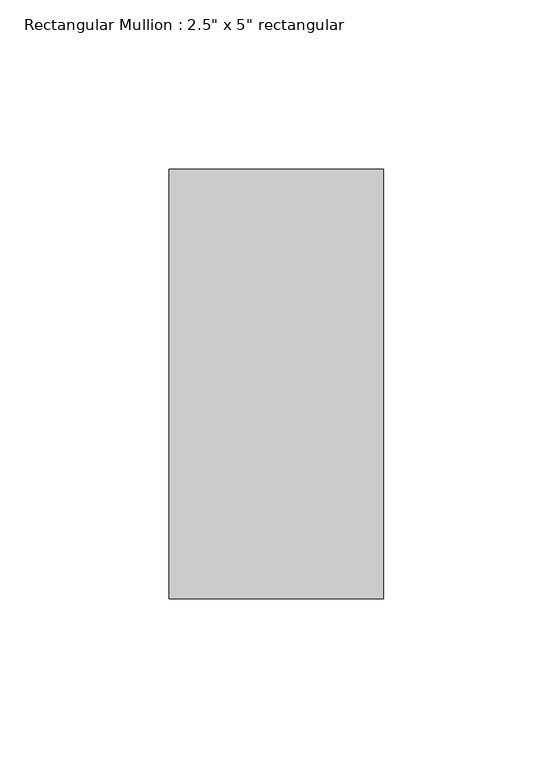
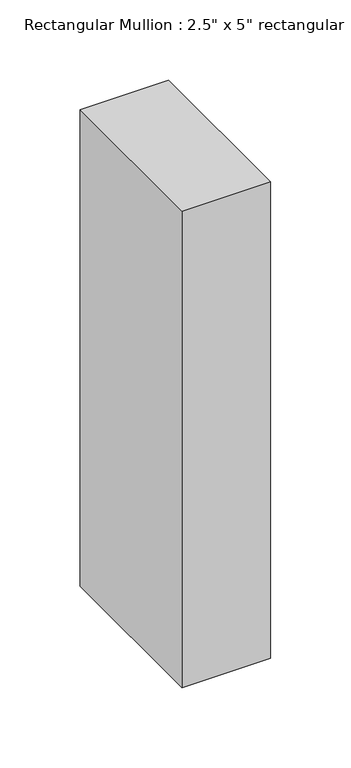
"""IFC4 building model written with IfcOpenShell, lengths in millimetres: member geometry."""

from ifc_helpers import new_model, si_unit, frame, origin, place, context, project, spatial, polyline, outline, extrude, source, transform, mapped, element, save


def member_af2f84b9(model_context):
    return source(origin(), model_context, "Body", "SweptSolid", [
        extrude(outline(polyline([(31.75, 63.5), (31.75, -63.5), (-31.75, -63.5), (-31.75, 63.5), (31.75, 63.5)])), frame((0.0, 0.0, -361.95), z_axis=(0.0, 0.0, 1.0), x_axis=(1.0, 0.0, 0.0)), (0.0, 0.0, 1.0), 361.95),
    ])


if __name__ == "__main__":
    model = new_model("IFC4")
    model_context = context("Model", 3, world=origin())
    ifc_project = project(units=[si_unit("LENGTHUNIT", "METRE", prefix="MILLI")], contexts=[model_context])
    site = spatial("IfcSite", under=ifc_project)
    building = spatial("IfcBuilding", under=site)
    placement = place(None, origin())
    member_shape = member_af2f84b9(model_context)
    element("IfcMember", 1, ObjectType="Rectangular Mullion : 2.5\" x 5\" rectangular", at=placement, inside=building, context=model_context, shape_type="MappedRepresentation", body=[
        mapped(member_shape, transform((0.0, 0.0, 0.0), x_axis=(1.0, 0.0, 0.0), y_axis=(0.0, 1.0, 0.0), z_axis=(0.0, 0.0, 1.0))),
    ])
    save(model, "model.ifc")

# Revit data of these elements
# Type "Rectangular Mullion : 2.5\" x 5\" rectangular"
#   built-in parameter 1007304 = 0.416667 (stored number, unit not read)
#   built-in parameter 1007301 = 0.104167 (stored number, unit not read)
#   built-in parameter 1007300 = 0.104167 (stored number, unit not read)
# Element 1 (IfcMember, "Rectangular Mullion : 2.5\" x 5\" rectangular")
#   Materials on its faces: "Aluminum"
# Materials
#   "Aluminum": class "Metal", colour RGB 247 247 247, transparency 0, Description = "Aluminum 6061", Cost = 0
